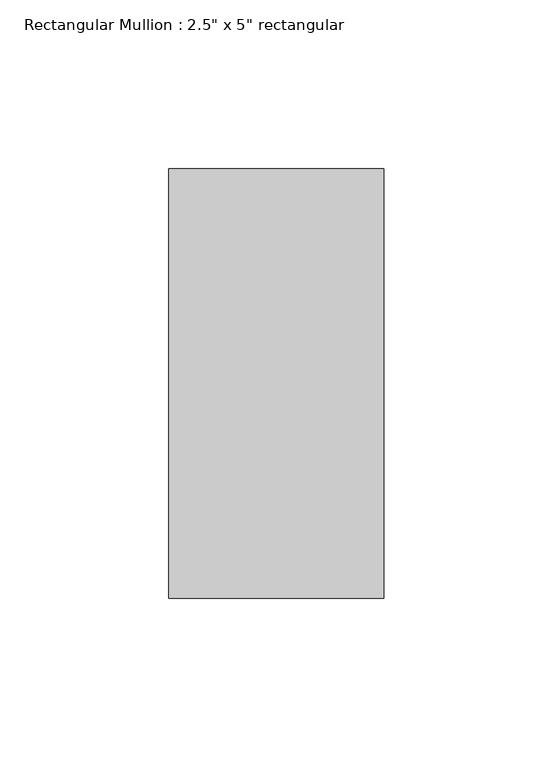
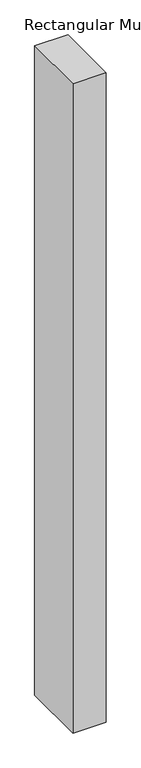
"""IFC4 building model written with IfcOpenShell, lengths in millimetres: member geometry."""

from ifc_helpers import new_model, si_unit, frame, origin, place, context, project, spatial, polyline, outline, extrude, source, transform, mapped, element, save


def member_640288a7(model_context):
    return source(origin(), model_context, "Body", "SweptSolid", [
        extrude(outline(polyline([(31.75, 63.5), (31.75, -63.5), (-31.75, -63.5), (-31.75, 63.5), (31.75, 63.5)])), frame((0.0, 0.0, -1315.425758), z_axis=(0.0, 0.0, 1.0), x_axis=(1.0, 0.0, 0.0)), (0.0, 0.0, 1.0), 1315.425758),
    ])


if __name__ == "__main__":
    model = new_model("IFC4")
    model_context = context("Model", 3, world=origin())
    ifc_project = project(units=[si_unit("LENGTHUNIT", "METRE", prefix="MILLI")], contexts=[model_context])
    site = spatial("IfcSite", under=ifc_project)
    building = spatial("IfcBuilding", under=site)
    placement = place(None, origin())
    member_shape = member_640288a7(model_context)
    element("IfcMember", 1, ObjectType="Rectangular Mullion : 2.5\" x 5\" rectangular", at=placement, inside=building, context=model_context, shape_type="MappedRepresentation", body=[
        mapped(member_shape, transform((0.0, 0.0, 0.0), x_axis=(1.0, 0.0, 0.0), y_axis=(0.0, 1.0, 0.0), z_axis=(0.0, 0.0, 1.0))),
    ])
    save(model, "model.ifc")

# Revit data of these elements
# Type "Rectangular Mullion : 2.5\" x 5\" rectangular"
#   built-in parameter 1007304 = 0.416667 (stored number, unit not read)
#   built-in parameter 1007301 = 0.104167 (stored number, unit not read)
#   built-in parameter 1007300 = 0.104167 (stored number, unit not read)
# Element 1 (IfcMember, "Rectangular Mullion : 2.5\" x 5\" rectangular")
#   Materials on its faces: "Aluminum"
# Materials
#   "Aluminum": class "Metal", colour RGB 247 247 247, transparency 0, Description = "Aluminum 6061", Cost = 0
